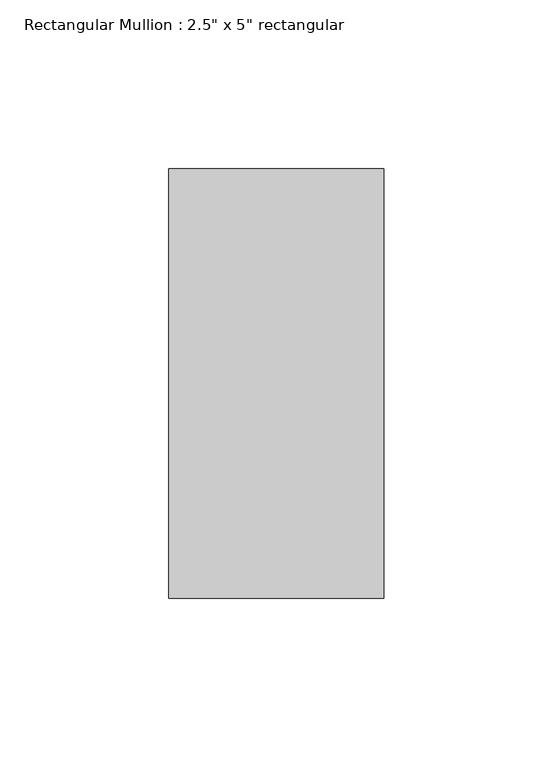
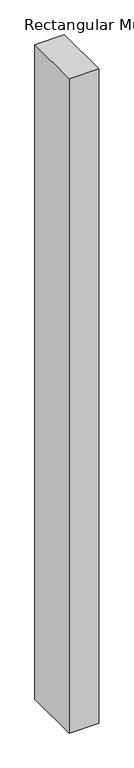
"""IFC4 building model written with IfcOpenShell, lengths in millimetres: member geometry."""

from ifc_helpers import new_model, si_unit, frame, origin, place, context, project, spatial, polyline, outline, extrude, source, transform, mapped, element, save


def member_b964ebf8(model_context):
    return source(origin(), model_context, "Body", "SweptSolid", [
        extrude(outline(polyline([(0.0, 63.5), (0.0, -63.5), (-63.5, -63.5), (-63.5, 63.5), (0.0, 63.5)])), frame((0.0, 0.0, -1485.9), z_axis=(0.0, 0.0, 1.0), x_axis=(1.0, 0.0, 0.0)), (0.0, 0.0, 1.0), 1485.9),
    ])


if __name__ == "__main__":
    model = new_model("IFC4")
    model_context = context("Model", 3, world=origin())
    ifc_project = project(units=[si_unit("LENGTHUNIT", "METRE", prefix="MILLI")], contexts=[model_context])
    site = spatial("IfcSite", under=ifc_project)
    building = spatial("IfcBuilding", under=site)
    placement = place(None, origin())
    member_shape = member_b964ebf8(model_context)
    element("IfcMember", 1, ObjectType="Rectangular Mullion : 2.5\" x 5\" rectangular", at=placement, inside=building, context=model_context, shape_type="MappedRepresentation", body=[
        mapped(member_shape, transform((0.0, 0.0, 0.0), x_axis=(1.0, 0.0, 0.0), y_axis=(0.0, 1.0, 0.0), z_axis=(0.0, 0.0, 1.0))),
    ])
    save(model, "model.ifc")

# Revit data of these elements
# Type "Rectangular Mullion : 2.5\" x 5\" rectangular"
#   built-in parameter 1007304 = 0.416667 (stored number, unit not read)
#   built-in parameter 1007301 = 0.104167 (stored number, unit not read)
#   built-in parameter 1007300 = 0.104167 (stored number, unit not read)
# Element 1 (IfcMember, "Rectangular Mullion : 2.5\" x 5\" rectangular")
#   Materials on its faces: "Aluminum"
# Materials
#   "Aluminum": class "Metal", colour RGB 247 247 247, transparency 0, Description = "Aluminum 6061", Cost = 0
